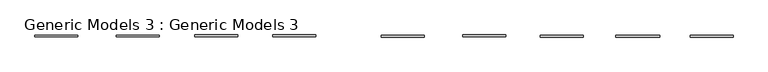
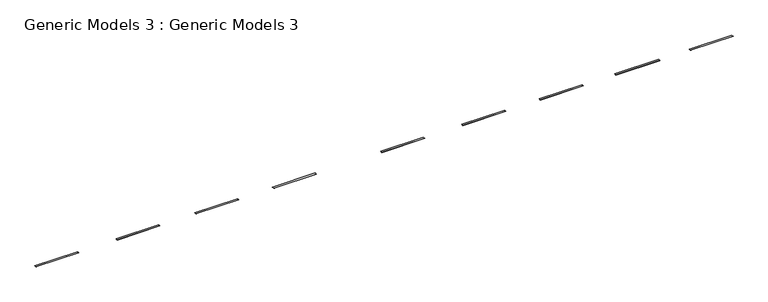
"""IFC4 building model written with IfcOpenShell, lengths in millimetres: proxy geometry, Generic Models 3 : Generic Models 3."""

from ifc_helpers import new_model, si_unit, frame, origin, place, context, project, spatial, polyline, outline, extrude, source, transform, mapped, element, save


def generic_models_3_generic_models_3_ad65571d(model_context):
    return source(origin(), model_context, "Body", "SweptSolid", [
        extrude(outline(polyline([(-51989.4631424, 4045.6553755), (-51989.4631424, 3994.8553755), (-53259.4631424, 3994.8553755), (-53259.4631424, 4045.6553755), (-51989.4631424, 4045.6553755)])), frame((0.0, 0.0, 449.9570313), z_axis=(0.0, 0.0, 1.0), x_axis=(1.0, 0.0, 0.0)), (0.0, 0.0, 1.0), 3.5784611),
        extrude(outline(polyline([(-49591.1403008, 4044.2925452), (-49591.1403008, 3993.4925452), (-50861.1403008, 3993.4925452), (-50861.1403008, 4044.2925452), (-49591.1403008, 4044.2925452)])), frame((0.0, 0.0, 449.9570313), z_axis=(0.0, 0.0, 1.0), x_axis=(1.0, 0.0, 0.0)), (0.0, 0.0, 1.0), 3.5784611),
        extrude(outline(polyline([(-47265.5162395, 4047.8313279), (-47265.5162395, 3997.0313279), (-48535.5162395, 3997.0313279), (-48535.5162395, 4047.8313279), (-47265.5162395, 4047.8313279)])), frame((0.0, 0.0, 449.9570313), z_axis=(0.0, 0.0, 1.0), x_axis=(1.0, 0.0, 0.0)), (0.0, 0.0, 1.0), 3.5784611),
        extrude(outline(polyline([(-44962.6691388, 4047.8313279), (-44962.6691388, 3990.6813279), (-46232.6691388, 3990.6813279), (-46232.6691388, 4047.8313279), (-44962.6691388, 4047.8313279)])), frame((0.0, 0.0, 449.9570313), z_axis=(0.0, 0.0, 1.0), x_axis=(1.0, 0.0, 0.0)), (0.0, 0.0, 1.0), 3.5784611),
        extrude(outline(polyline([(-41766.3609152, 4044.9101949), (-41766.3609152, 3987.7601949), (-43026.6088216, 3987.7601949), (-43026.6088216, 4044.9101949), (-41766.3609152, 4044.9101949)])), frame((0.0, 0.0, 449.9570313), z_axis=(0.0, 0.0, 1.0), x_axis=(1.0, 0.0, 0.0)), (0.0, 0.0, 1.0), 3.5784611),
        extrude(outline(polyline([(-39358.1980607, 4050.0131176), (-39358.1980607, 3992.8631176), (-40628.1980607, 3992.8631176), (-40628.1980607, 4050.0131176), (-39358.1980607, 4050.0131176)])), frame((0.0, 0.0, 449.9570313), z_axis=(0.0, 0.0, 1.0), x_axis=(1.0, 0.0, 0.0)), (0.0, 0.0, 1.0), 3.5784611),
        extrude(outline(polyline([(-37068.0710983, 4044.8105849), (-37068.0710983, 3987.6605849), (-38338.0710983, 3987.6605849), (-38338.0710983, 4044.8105849), (-37068.0710983, 4044.8105849)])), frame((0.0, 0.0, 449.9570313), z_axis=(0.0, 0.0, 1.0), x_axis=(1.0, 0.0, 0.0)), (0.0, 0.0, 1.0), 3.5784611),
        extrude(outline(polyline([(-34807.4710983, 4044.8105849), (-34807.4710983, 3987.6605849), (-36102.8710983, 3987.6605849), (-36102.8710983, 4044.8105849), (-34807.4710983, 4044.8105849)])), frame((0.0, 0.0, 449.9570313), z_axis=(0.0, 0.0, 1.0), x_axis=(1.0, 0.0, 0.0)), (0.0, 0.0, 1.0), 3.5784611),
        extrude(outline(polyline([(-32637.1571981, 4044.8105849), (-32637.1571981, 3987.6605849), (-33900.8071981, 3987.6605849), (-33900.8071981, 4044.8105849), (-32637.1571981, 4044.8105849)])), frame((0.0, 0.0, 449.9570313), z_axis=(0.0, 0.0, 1.0), x_axis=(1.0, 0.0, 0.0)), (0.0, 0.0, 1.0), 3.5784611),
    ])


if __name__ == "__main__":
    model = new_model("IFC4")
    model_context = context("Model", 3, world=origin())
    ifc_project = project(units=[si_unit("LENGTHUNIT", "METRE", prefix="MILLI")], contexts=[model_context])
    site = spatial("IfcSite", under=ifc_project)
    building = spatial("IfcBuilding", under=site)
    placement = place(None, origin())
    generic_models_3_generic_models_3_shape = generic_models_3_generic_models_3_ad65571d(model_context)
    element("IfcBuildingElementProxy", 1, Name="Generic Models 3 : Generic Models 3", ObjectType="Generic Models 3 : Generic Models 3", at=placement, inside=building, context=model_context, shape_type="MappedRepresentation", body=[
        mapped(generic_models_3_generic_models_3_shape, transform((0.0, 0.0, 0.0), x_axis=(1.0, 0.0, 0.0), y_axis=(0.0, 1.0, 0.0), z_axis=(0.0, 0.0, 1.0))),
    ])
    save(model, "model.ifc")
